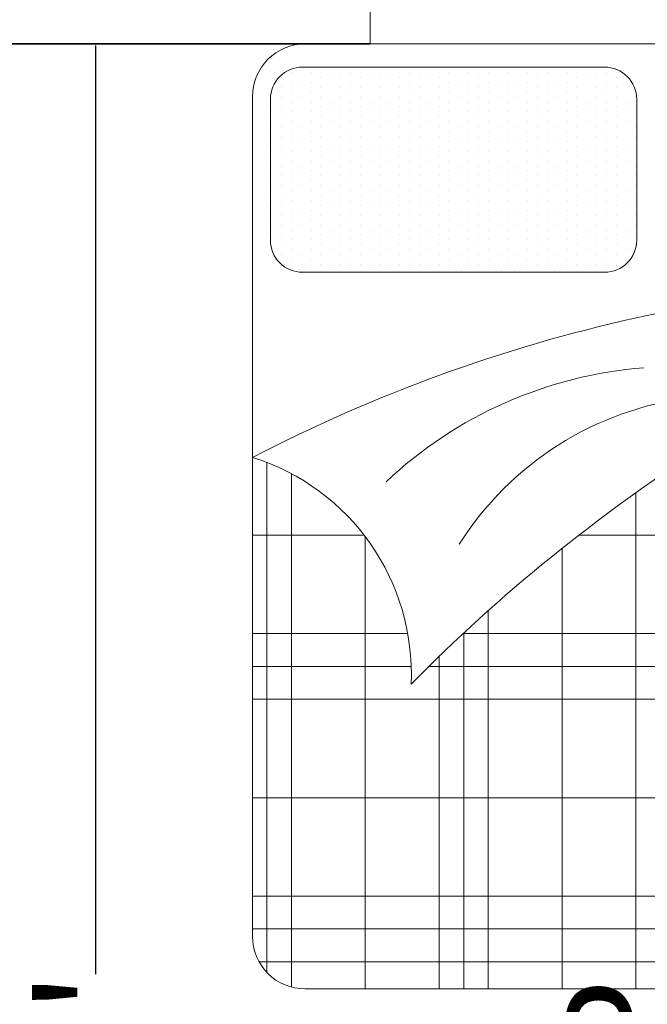
# Model space of a CAD drawing. Units: inches. Extents: x -269 to 4574, y -694 to 313.
# Tile 12 of 19: x 302 to 357, y -74 to 11. Entities that reach past the tile are written whole.
import ezdxf

# ---------------------------------------------------------------- set-up
doc = ezdxf.new("R2010")
doc.units = ezdxf.units.IN
doc.header["$MEASUREMENT"] = 0
for name, color, linetype, lineweight in [('A-FURN', 2, 'Continuous', 18), ('DIMENSION', 5, 'Continuous', 18), ('WALL', 1, 'Continuous', 35), ('WINDOWS', 2, 'Continuous', 18)]:
    doc.layers.add(name, color=color, linetype=linetype, lineweight=lineweight)
doc.dimstyles.get("Standard").update_dxf_attribs({"dimtxt": 10, "dimasz": 0.18, "dimexe": 0.18, "dimexo": 0.0625, "dimgap": 0.09, "dimtad": 0, "dimdec": 1, "dimzin": 0, "dimdsep": 46, "dimlunit": 3, "dimtxsty": 'Standard', "dimcen": 0.09, "dimclrt": 7, "dimadec": 0, "dimazin": 0, "dimtfac": 1, "dimtdec": 1, "dimtofl": 0, "dimtmove": 0, "dimatfit": 3, "dimfxl": 1, "dimtolj": 1, "dimtzin": 0, "dimarcsym": 0})

# ---------------------------------------------------------------- blocks, each defined once
blk = doc.blocks.new('*X12')
at = {"color": 0}
for p, q in [((266.25, 456.9375), (266.25, 456.9375)), ((266.4375, 457.03125), (266.4375, 457.03125)), ((266.625, 456.9375), (266.625, 456.9375)), ((266.8125, 457.03125), (266.8125, 457.03125)), ((267, 456.9375), (267, 456.9375)), ((267.1875, 457.03125), (267.1875, 457.03125)), ((267.375, 456.9375), (267.375, 456.9375)), ((267.5625, 457.03125), (267.5625, 457.03125)), ((267.75, 456.9375), (267.75, 456.9375)), ((267.9375, 457.03125), (267.9375, 457.03125)), ((268.125, 456.9375), (268.125, 456.9375)), ((268.3125, 457.03125), (268.3125, 457.03125)), ((268.5, 456.9375), (268.5, 456.9375)), ((268.6875, 457.03125), (268.6875, 457.03125)), ((268.875, 456.9375), (268.875, 456.9375)), ((269.0625, 457.03125), (269.0625, 457.03125)), ((269.25, 456.9375), (269.25, 456.9375)), ((269.4375, 457.03125), (269.4375, 457.03125)), ((269.625, 456.9375), (269.625, 456.9375)), ((269.8125, 457.03125), (269.8125, 457.03125)), ((270, 456.9375), (270, 456.9375)), ((270.1875, 457.03125), (270.1875, 457.03125)), ((270.375, 456.9375), (270.375, 456.9375)), ((270.5625, 457.03125), (270.5625, 457.03125)), ((270.75, 456.9375), (270.75, 456.9375)), ((270.9375, 457.03125), (270.9375, 457.03125)), ((271.125, 456.9375), (271.125, 456.9375)), ((271.3125, 457.03125), (271.3125, 457.03125)), ((271.5, 456.9375), (271.5, 456.9375)), ((271.6875, 457.03125), (271.6875, 457.03125)), ((271.875, 456.9375), (271.875, 456.9375)), ((272.0625, 457.03125), (272.0625, 457.03125)), ((272.25, 456.9375), (272.25, 456.9375)), ((266.0625, 456.84375), (266.0625, 456.84375)), ((266.25, 456.75), (266.25, 456.75)), ((266.4375, 456.84375), (266.4375, 456.84375)), ((266.625, 456.75), (266.625, 456.75)), ((266.8125, 456.84375), (266.8125, 456.84375)), ((267, 456.75), (267, 456.75)), ((267.1875, 456.84375), (267.1875, 456.84375)), ((267.375, 456.75), (267.375, 456.75)), ((267.5625, 456.84375), (267.5625, 456.84375)), ((267.75, 456.75), (267.75, 456.75)), ((267.9375, 456.84375), (267.9375, 456.84375)), ((268.125, 456.75), (268.125, 456.75)), ((268.3125, 456.84375), (268.3125, 456.84375)), ((268.5, 456.75), (268.5, 456.75)), ((268.6875, 456.84375), (268.6875, 456.84375)), ((268.875, 456.75), (268.875, 456.75)), ((269.0625, 456.84375), (269.0625, 456.84375)), ((269.25, 456.75), (269.25, 456.75)), ((269.4375, 456.84375), (269.4375, 456.84375)), ((269.625, 456.75), (269.625, 456.75)), ((269.8125, 456.84375), (269.8125, 456.84375)), ((270, 456.75), (270, 456.75)), ((270.1875, 456.84375), (270.1875, 456.84375)), ((270.375, 456.75), (270.375, 456.75)), ((270.5625, 456.84375), (270.5625, 456.84375)), ((270.75, 456.75), (270.75, 456.75)), ((270.9375, 456.84375), (270.9375, 456.84375)), ((271.125, 456.75), (271.125, 456.75)), ((271.3125, 456.84375), (271.3125, 456.84375)), ((271.5, 456.75), (271.5, 456.75)), ((271.6875, 456.84375), (271.6875, 456.84375)), ((271.875, 456.75), (271.875, 456.75)), ((272.0625, 456.84375), (272.0625, 456.84375)), ((272.25, 456.75), (272.25, 456.75)), ((272.4375, 456.84375), (272.4375, 456.84375)), ((272.625, 456.75), (272.625, 456.75)), ((265.875, 456.5625), (265.875, 456.5625)), ((266.0625, 456.65625), (266.0625, 456.65625)), ((266.25, 456.5625), (266.25, 456.5625)), ((266.4375, 456.65625), (266.4375, 456.65625)), ((266.625, 456.5625), (266.625, 456.5625)), ((266.8125, 456.65625), (266.8125, 456.65625)), ((267, 456.5625), (267, 456.5625)), ((267.1875, 456.65625), (267.1875, 456.65625)), ((267.375, 456.5625), (267.375, 456.5625)), ((267.5625, 456.65625), (267.5625, 456.65625)), ((267.75, 456.5625), (267.75, 456.5625)), ((267.9375, 456.65625), (267.9375, 456.65625)), ((268.125, 456.5625), (268.125, 456.5625)), ((268.3125, 456.65625), (268.3125, 456.65625)), ((268.5, 456.5625), (268.5, 456.5625)), ((268.6875, 456.65625), (268.6875, 456.65625)), ((268.875, 456.5625), (268.875, 456.5625)), ((269.0625, 456.65625), (269.0625, 456.65625)), ((269.25, 456.5625), (269.25, 456.5625)), ((269.4375, 456.65625), (269.4375, 456.65625)), ((269.625, 456.5625), (269.625, 456.5625)), ((269.8125, 456.65625), (269.8125, 456.65625)), ((270, 456.5625), (270, 456.5625)), ((270.1875, 456.65625), (270.1875, 456.65625)), ((270.375, 456.5625), (270.375, 456.5625)), ((270.5625, 456.65625), (270.5625, 456.65625)), ((270.75, 456.5625), (270.75, 456.5625)), ((270.9375, 456.65625), (270.9375, 456.65625)), ((271.125, 456.5625), (271.125, 456.5625)), ((271.3125, 456.65625), (271.3125, 456.65625)), ((271.5, 456.5625), (271.5, 456.5625)), ((271.6875, 456.65625), (271.6875, 456.65625)), ((271.875, 456.5625), (271.875, 456.5625)), ((272.0625, 456.65625), (272.0625, 456.65625)), ((272.25, 456.5625), (272.25, 456.5625)), ((272.4375, 456.65625), (272.4375, 456.65625)), ((272.625, 456.5625), (272.625, 456.5625)), ((265.875, 456.375), (265.875, 456.375)), ((266.0625, 456.46875), (266.0625, 456.46875)), ((266.25, 456.375), (266.25, 456.375)), ((266.4375, 456.46875), (266.4375, 456.46875)), ((266.625, 456.375), (266.625, 456.375)), ((266.8125, 456.46875), (266.8125, 456.46875)), ((267, 456.375), (267, 456.375)), ((267.1875, 456.46875), (267.1875, 456.46875)), ((267.375, 456.375), (267.375, 456.375)), ((267.5625, 456.46875), (267.5625, 456.46875)), ((267.75, 456.375), (267.75, 456.375)), ((267.9375, 456.46875), (267.9375, 456.46875)), ((268.125, 456.375), (268.125, 456.375)), ((268.3125, 456.46875), (268.3125, 456.46875)), ((268.5, 456.375), (268.5, 456.375)), ((268.6875, 456.46875), (268.6875, 456.46875)), ((268.875, 456.375), (268.875, 456.375)), ((269.0625, 456.46875), (269.0625, 456.46875)), ((269.25, 456.375), (269.25, 456.375)), ((269.4375, 456.46875), (269.4375, 456.46875)), ((269.625, 456.375), (269.625, 456.375)), ((269.8125, 456.46875), (269.8125, 456.46875)), ((270, 456.375), (270, 456.375)), ((270.1875, 456.46875), (270.1875, 456.46875)), ((270.375, 456.375), (270.375, 456.375)), ((270.5625, 456.46875), (270.5625, 456.46875)), ((270.75, 456.375), (270.75, 456.375)), ((270.9375, 456.46875), (270.9375, 456.46875)), ((271.125, 456.375), (271.125, 456.375)), ((271.3125, 456.46875), (271.3125, 456.46875)), ((271.5, 456.375), (271.5, 456.375)), ((271.6875, 456.46875), (271.6875, 456.46875)), ((271.875, 456.375), (271.875, 456.375)), ((272.0625, 456.46875), (272.0625, 456.46875)), ((272.25, 456.375), (272.25, 456.375)), ((272.4375, 456.46875), (272.4375, 456.46875)), ((272.625, 456.375), (272.625, 456.375)), ((272.8125, 456.46875), (272.8125, 456.46875)), ((265.875, 456.1875), (265.875, 456.1875)), ((266.0625, 456.28125), (266.0625, 456.28125)), ((266.25, 456.1875), (266.25, 456.1875)), ((266.4375, 456.28125), (266.4375, 456.28125)), ((266.625, 456.1875), (266.625, 456.1875)), ((266.8125, 456.28125), (266.8125, 456.28125)), ((267, 456.1875), (267, 456.1875)), ((267.1875, 456.28125), (267.1875, 456.28125)), ((267.375, 456.1875), (267.375, 456.1875)), ((267.5625, 456.28125), (267.5625, 456.28125)), ((267.75, 456.1875), (267.75, 456.1875)), ((267.9375, 456.28125), (267.9375, 456.28125)), ((268.125, 456.1875), (268.125, 456.1875)), ((268.3125, 456.28125), (268.3125, 456.28125)), ((268.5, 456.1875), (268.5, 456.1875)), ((268.6875, 456.28125), (268.6875, 456.28125)), ((268.875, 456.1875), (268.875, 456.1875)), ((269.0625, 456.28125), (269.0625, 456.28125)), ((269.25, 456.1875), (269.25, 456.1875)), ((269.4375, 456.28125), (269.4375, 456.28125)), ((269.625, 456.1875), (269.625, 456.1875)), ((269.8125, 456.28125), (269.8125, 456.28125)), ((270, 456.1875), (270, 456.1875)), ((270.1875, 456.28125), (270.1875, 456.28125)), ((270.375, 456.1875), (270.375, 456.1875)), ((270.5625, 456.28125), (270.5625, 456.28125)), ((270.75, 456.1875), (270.75, 456.1875)), ((270.9375, 456.28125), (270.9375, 456.28125)), ((271.125, 456.1875), (271.125, 456.1875)), ((271.3125, 456.28125), (271.3125, 456.28125)), ((271.5, 456.1875), (271.5, 456.1875)), ((271.6875, 456.28125), (271.6875, 456.28125)), ((271.875, 456.1875), (271.875, 456.1875)), ((272.0625, 456.28125), (272.0625, 456.28125)), ((272.25, 456.1875), (272.25, 456.1875)), ((272.4375, 456.28125), (272.4375, 456.28125)), ((272.625, 456.1875), (272.625, 456.1875)), ((272.8125, 456.28125), (272.8125, 456.28125)), ((265.875, 456), (265.875, 456)), ((266.0625, 456.09375), (266.0625, 456.09375)), ((266.25, 456), (266.25, 456)), ((266.4375, 456.09375), (266.4375, 456.09375)), ((266.625, 456), (266.625, 456)), ((266.8125, 456.09375), (266.8125, 456.09375)), ((267, 456), (267, 456)), ((267.1875, 456.09375), (267.1875, 456.09375)), ((267.375, 456), (267.375, 456)), ((267.5625, 456.09375), (267.5625, 456.09375)), ((267.75, 456), (267.75, 456)), ((267.9375, 456.09375), (267.9375, 456.09375)), ((268.125, 456), (268.125, 456)), ((268.3125, 456.09375), (268.3125, 456.09375)), ((268.5, 456), (268.5, 456)), ((268.6875, 456.09375), (268.6875, 456.09375)), ((268.875, 456), (268.875, 456)), ((269.0625, 456.09375), (269.0625, 456.09375)), ((269.25, 456), (269.25, 456)), ((269.4375, 456.09375), (269.4375, 456.09375)), ((269.625, 456), (269.625, 456)), ((269.8125, 456.09375), (269.8125, 456.09375)), ((270, 456), (270, 456)), ((270.1875, 456.09375), (270.1875, 456.09375)), ((270.375, 456), (270.375, 456)), ((270.5625, 456.09375), (270.5625, 456.09375)), ((270.75, 456), (270.75, 456)), ((270.9375, 456.09375), (270.9375, 456.09375)), ((271.125, 456), (271.125, 456)), ((271.3125, 456.09375), (271.3125, 456.09375)), ((271.5, 456), (271.5, 456)), ((271.6875, 456.09375), (271.6875, 456.09375)), ((271.875, 456), (271.875, 456)), ((272.0625, 456.09375), (272.0625, 456.09375)), ((272.25, 456), (272.25, 456)), ((272.4375, 456.09375), (272.4375, 456.09375)), ((272.625, 456), (272.625, 456)), ((272.8125, 456.09375), (272.8125, 456.09375)), ((265.875, 455.8125), (265.875, 455.8125)), ((266.0625, 455.90625), (266.0625, 455.90625)), ((266.25, 455.8125), (266.25, 455.8125)), ((266.4375, 455.90625), (266.4375, 455.90625)), ((266.625, 455.8125), (266.625, 455.8125)), ((266.8125, 455.90625), (266.8125, 455.90625)), ((267, 455.8125), (267, 455.8125)), ((267.1875, 455.90625), (267.1875, 455.90625)), ((267.375, 455.8125), (267.375, 455.8125)), ((267.5625, 455.90625), (267.5625, 455.90625)), ((267.75, 455.8125), (267.75, 455.8125)), ((267.9375, 455.90625), (267.9375, 455.90625)), ((268.125, 455.8125), (268.125, 455.8125)), ((268.3125, 455.90625), (268.3125, 455.90625)), ((268.5, 455.8125), (268.5, 455.8125)), ((268.6875, 455.90625), (268.6875, 455.90625)), ((268.875, 455.8125), (268.875, 455.8125)), ((269.0625, 455.90625), (269.0625, 455.90625)), ((269.25, 455.8125), (269.25, 455.8125)), ((269.4375, 455.90625), (269.4375, 455.90625)), ((269.625, 455.8125), (269.625, 455.8125)), ((269.8125, 455.90625), (269.8125, 455.90625)), ((270, 455.8125), (270, 455.8125)), ((270.1875, 455.90625), (270.1875, 455.90625)), ((270.375, 455.8125), (270.375, 455.8125)), ((270.5625, 455.90625), (270.5625, 455.90625)), ((270.75, 455.8125), (270.75, 455.8125)), ((270.9375, 455.90625), (270.9375, 455.90625)), ((271.125, 455.8125), (271.125, 455.8125)), ((271.3125, 455.90625), (271.3125, 455.90625)), ((271.5, 455.8125), (271.5, 455.8125)), ((271.6875, 455.90625), (271.6875, 455.90625)), ((271.875, 455.8125), (271.875, 455.8125)), ((272.0625, 455.90625), (272.0625, 455.90625)), ((272.25, 455.8125), (272.25, 455.8125)), ((272.4375, 455.90625), (272.4375, 455.90625)), ((272.625, 455.8125), (272.625, 455.8125)), ((272.8125, 455.90625), (272.8125, 455.90625)), ((265.875, 455.625), (265.875, 455.625)), ((266.0625, 455.71875), (266.0625, 455.71875)), ((266.25, 455.625), (266.25, 455.625)), ((266.4375, 455.71875), (266.4375, 455.71875)), ((266.625, 455.625), (266.625, 455.625)), ((266.8125, 455.71875), (266.8125, 455.71875)), ((267, 455.625), (267, 455.625)), ((267.1875, 455.71875), (267.1875, 455.71875)), ((267.375, 455.625), (267.375, 455.625)), ((267.5625, 455.71875), (267.5625, 455.71875)), ((267.75, 455.625), (267.75, 455.625)), ((267.9375, 455.71875), (267.9375, 455.71875)), ((268.125, 455.625), (268.125, 455.625)), ((268.3125, 455.71875), (268.3125, 455.71875)), ((268.5, 455.625), (268.5, 455.625)), ((268.6875, 455.71875), (268.6875, 455.71875)), ((268.875, 455.625), (268.875, 455.625)), ((269.0625, 455.71875), (269.0625, 455.71875)), ((269.25, 455.625), (269.25, 455.625)), ((269.4375, 455.71875), (269.4375, 455.71875)), ((269.625, 455.625), (269.625, 455.625)), ((269.8125, 455.71875), (269.8125, 455.71875)), ((270, 455.625), (270, 455.625)), ((270.1875, 455.71875), (270.1875, 455.71875)), ((270.375, 455.625), (270.375, 455.625)), ((270.5625, 455.71875), (270.5625, 455.71875)), ((270.75, 455.625), (270.75, 455.625)), ((270.9375, 455.71875), (270.9375, 455.71875)), ((271.125, 455.625), (271.125, 455.625)), ((271.3125, 455.71875), (271.3125, 455.71875)), ((271.5, 455.625), (271.5, 455.625)), ((271.6875, 455.71875), (271.6875, 455.71875)), ((271.875, 455.625), (271.875, 455.625)), ((272.0625, 455.71875), (272.0625, 455.71875)), ((272.25, 455.625), (272.25, 455.625)), ((272.4375, 455.71875), (272.4375, 455.71875)), ((272.625, 455.625), (272.625, 455.625)), ((272.8125, 455.71875), (272.8125, 455.71875)), ((265.875, 455.4375), (265.875, 455.4375)), ((266.0625, 455.53125), (266.0625, 455.53125)), ((266.25, 455.4375), (266.25, 455.4375)), ((266.4375, 455.53125), (266.4375, 455.53125)), ((266.625, 455.4375), (266.625, 455.4375)), ((266.8125, 455.53125), (266.8125, 455.53125)), ((267, 455.4375), (267, 455.4375)), ((267.1875, 455.53125), (267.1875, 455.53125)), ((267.375, 455.4375), (267.375, 455.4375)), ((267.5625, 455.53125), (267.5625, 455.53125)), ((267.75, 455.4375), (267.75, 455.4375)), ((267.9375, 455.53125), (267.9375, 455.53125)), ((268.125, 455.4375), (268.125, 455.4375)), ((268.3125, 455.53125), (268.3125, 455.53125)), ((268.5, 455.4375), (268.5, 455.4375)), ((268.6875, 455.53125), (268.6875, 455.53125)), ((268.875, 455.4375), (268.875, 455.4375)), ((269.0625, 455.53125), (269.0625, 455.53125)), ((269.25, 455.4375), (269.25, 455.4375)), ((269.4375, 455.53125), (269.4375, 455.53125)), ((269.625, 455.4375), (269.625, 455.4375)), ((269.8125, 455.53125), (269.8125, 455.53125)), ((270, 455.4375), (270, 455.4375)), ((270.1875, 455.53125), (270.1875, 455.53125)), ((270.375, 455.4375), (270.375, 455.4375)), ((270.5625, 455.53125), (270.5625, 455.53125)), ((270.75, 455.4375), (270.75, 455.4375)), ((270.9375, 455.53125), (270.9375, 455.53125)), ((271.125, 455.4375), (271.125, 455.4375)), ((271.3125, 455.53125), (271.3125, 455.53125)), ((271.5, 455.4375), (271.5, 455.4375)), ((271.6875, 455.53125), (271.6875, 455.53125)), ((271.875, 455.4375), (271.875, 455.4375)), ((272.0625, 455.53125), (272.0625, 455.53125)), ((272.25, 455.4375), (272.25, 455.4375)), ((272.4375, 455.53125), (272.4375, 455.53125)), ((272.625, 455.4375), (272.625, 455.4375)), ((272.8125, 455.53125), (272.8125, 455.53125)), ((265.875, 455.25), (265.875, 455.25)), ((266.0625, 455.34375), (266.0625, 455.34375)), ((266.25, 455.25), (266.25, 455.25)), ((266.4375, 455.34375), (266.4375, 455.34375)), ((266.625, 455.25), (266.625, 455.25)), ((266.8125, 455.34375), (266.8125, 455.34375)), ((267, 455.25), (267, 455.25)), ((267.1875, 455.34375), (267.1875, 455.34375)), ((267.375, 455.25), (267.375, 455.25)), ((267.5625, 455.34375), (267.5625, 455.34375)), ((267.75, 455.25), (267.75, 455.25)), ((267.9375, 455.34375), (267.9375, 455.34375)), ((268.125, 455.25), (268.125, 455.25)), ((268.3125, 455.34375), (268.3125, 455.34375)), ((268.5, 455.25), (268.5, 455.25)), ((268.6875, 455.34375), (268.6875, 455.34375)), ((268.875, 455.25), (268.875, 455.25)), ((269.0625, 455.34375), (269.0625, 455.34375)), ((269.25, 455.25), (269.25, 455.25)), ((269.4375, 455.34375), (269.4375, 455.34375)), ((269.625, 455.25), (269.625, 455.25)), ((269.8125, 455.34375), (269.8125, 455.34375)), ((270, 455.25), (270, 455.25)), ((270.1875, 455.34375), (270.1875, 455.34375)), ((270.375, 455.25), (270.375, 455.25)), ((270.5625, 455.34375), (270.5625, 455.34375)), ((270.75, 455.25), (270.75, 455.25)), ((270.9375, 455.34375), (270.9375, 455.34375)), ((271.125, 455.25), (271.125, 455.25)), ((271.3125, 455.34375), (271.3125, 455.34375)), ((271.5, 455.25), (271.5, 455.25)), ((271.6875, 455.34375), (271.6875, 455.34375)), ((271.875, 455.25), (271.875, 455.25)), ((272.0625, 455.34375), (272.0625, 455.34375)), ((272.25, 455.25), (272.25, 455.25)), ((272.4375, 455.34375), (272.4375, 455.34375)), ((272.625, 455.25), (272.625, 455.25)), ((272.8125, 455.34375), (272.8125, 455.34375)), ((265.875, 455.0625), (265.875, 455.0625)), ((266.0625, 455.15625), (266.0625, 455.15625)), ((266.25, 455.0625), (266.25, 455.0625)), ((266.4375, 455.15625), (266.4375, 455.15625)), ((266.625, 455.0625), (266.625, 455.0625)), ((266.8125, 455.15625), (266.8125, 455.15625)), ((267, 455.0625), (267, 455.0625)), ((267.1875, 455.15625), (267.1875, 455.15625)), ((267.375, 455.0625), (267.375, 455.0625)), ((267.5625, 455.15625), (267.5625, 455.15625)), ((267.75, 455.0625), (267.75, 455.0625)), ((267.9375, 455.15625), (267.9375, 455.15625)), ((268.125, 455.0625), (268.125, 455.0625)), ((268.3125, 455.15625), (268.3125, 455.15625)), ((268.5, 455.0625), (268.5, 455.0625)), ((268.6875, 455.15625), (268.6875, 455.15625)), ((268.875, 455.0625), (268.875, 455.0625)), ((269.0625, 455.15625), (269.0625, 455.15625)), ((269.25, 455.0625), (269.25, 455.0625)), ((269.4375, 455.15625), (269.4375, 455.15625)), ((269.625, 455.0625), (269.625, 455.0625)), ((269.8125, 455.15625), (269.8125, 455.15625)), ((270, 455.0625), (270, 455.0625)), ((270.1875, 455.15625), (270.1875, 455.15625)), ((270.375, 455.0625), (270.375, 455.0625)), ((270.5625, 455.15625), (270.5625, 455.15625)), ((270.75, 455.0625), (270.75, 455.0625)), ((270.9375, 455.15625), (270.9375, 455.15625)), ((271.125, 455.0625), (271.125, 455.0625)), ((271.3125, 455.15625), (271.3125, 455.15625)), ((271.5, 455.0625), (271.5, 455.0625)), ((271.6875, 455.15625), (271.6875, 455.15625)), ((271.875, 455.0625), (271.875, 455.0625)), ((272.0625, 455.15625), (272.0625, 455.15625)), ((272.25, 455.0625), (272.25, 455.0625)), ((272.4375, 455.15625), (272.4375, 455.15625)), ((272.625, 455.0625), (272.625, 455.0625)), ((272.8125, 455.15625), (272.8125, 455.15625)), ((265.875, 454.875), (265.875, 454.875)), ((266.0625, 454.96875), (266.0625, 454.96875)), ((266.25, 454.875), (266.25, 454.875)), ((266.4375, 454.96875), (266.4375, 454.96875)), ((266.625, 454.875), (266.625, 454.875)), ((266.8125, 454.96875), (266.8125, 454.96875)), ((267, 454.875), (267, 454.875)), ((267.1875, 454.96875), (267.1875, 454.96875)), ((267.375, 454.875), (267.375, 454.875)), ((267.5625, 454.96875), (267.5625, 454.96875)), ((267.75, 454.875), (267.75, 454.875)), ((267.9375, 454.96875), (267.9375, 454.96875)), ((268.125, 454.875), (268.125, 454.875)), ((268.3125, 454.96875), (268.3125, 454.96875)), ((268.5, 454.875), (268.5, 454.875)), ((268.6875, 454.96875), (268.6875, 454.96875)), ((268.875, 454.875), (268.875, 454.875)), ((269.0625, 454.96875), (269.0625, 454.96875)), ((269.25, 454.875), (269.25, 454.875)), ((269.4375, 454.96875), (269.4375, 454.96875)), ((269.625, 454.875), (269.625, 454.875)), ((269.8125, 454.96875), (269.8125, 454.96875)), ((270, 454.875), (270, 454.875)), ((270.1875, 454.96875), (270.1875, 454.96875)), ((270.375, 454.875), (270.375, 454.875)), ((270.5625, 454.96875), (270.5625, 454.96875)), ((270.75, 454.875), (270.75, 454.875)), ((270.9375, 454.96875), (270.9375, 454.96875)), ((271.125, 454.875), (271.125, 454.875)), ((271.3125, 454.96875), (271.3125, 454.96875)), ((271.5, 454.875), (271.5, 454.875)), ((271.6875, 454.96875), (271.6875, 454.96875)), ((271.875, 454.875), (271.875, 454.875)), ((272.0625, 454.96875), (272.0625, 454.96875)), ((272.25, 454.875), (272.25, 454.875)), ((272.4375, 454.96875), (272.4375, 454.96875)), ((272.625, 454.875), (272.625, 454.875)), ((272.8125, 454.96875), (272.8125, 454.96875)), ((265.875, 454.6875), (265.875, 454.6875)), ((266.0625, 454.78125), (266.0625, 454.78125)), ((266.25, 454.6875), (266.25, 454.6875)), ((266.4375, 454.78125), (266.4375, 454.78125)), ((266.625, 454.6875), (266.625, 454.6875)), ((266.8125, 454.78125), (266.8125, 454.78125)), ((267, 454.6875), (267, 454.6875)), ((267.1875, 454.78125), (267.1875, 454.78125)), ((267.375, 454.6875), (267.375, 454.6875)), ((267.5625, 454.78125), (267.5625, 454.78125)), ((267.75, 454.6875), (267.75, 454.6875)), ((267.9375, 454.78125), (267.9375, 454.78125)), ((268.125, 454.6875), (268.125, 454.6875)), ((268.3125, 454.78125), (268.3125, 454.78125)), ((268.5, 454.6875), (268.5, 454.6875)), ((268.6875, 454.78125), (268.6875, 454.78125)), ((268.875, 454.6875), (268.875, 454.6875)), ((269.0625, 454.78125), (269.0625, 454.78125)), ((269.25, 454.6875), (269.25, 454.6875)), ((269.4375, 454.78125), (269.4375, 454.78125)), ((269.625, 454.6875), (269.625, 454.6875)), ((269.8125, 454.78125), (269.8125, 454.78125)), ((270, 454.6875), (270, 454.6875)), ((270.1875, 454.78125), (270.1875, 454.78125)), ((270.375, 454.6875), (270.375, 454.6875)), ((270.5625, 454.78125), (270.5625, 454.78125)), ((270.75, 454.6875), (270.75, 454.6875)), ((270.9375, 454.78125), (270.9375, 454.78125)), ((271.125, 454.6875), (271.125, 454.6875)), ((271.3125, 454.78125), (271.3125, 454.78125)), ((271.5, 454.6875), (271.5, 454.6875)), ((271.6875, 454.78125), (271.6875, 454.78125)), ((271.875, 454.6875), (271.875, 454.6875)), ((272.0625, 454.78125), (272.0625, 454.78125)), ((272.25, 454.6875), (272.25, 454.6875)), ((272.4375, 454.78125), (272.4375, 454.78125)), ((272.625, 454.6875), (272.625, 454.6875)), ((272.8125, 454.78125), (272.8125, 454.78125)), ((265.875, 454.5), (265.875, 454.5)), ((266.0625, 454.59375), (266.0625, 454.59375)), ((266.25, 454.5), (266.25, 454.5)), ((266.4375, 454.59375), (266.4375, 454.59375)), ((266.625, 454.5), (266.625, 454.5)), ((266.8125, 454.59375), (266.8125, 454.59375)), ((267, 454.5), (267, 454.5)), ((267.1875, 454.59375), (267.1875, 454.59375)), ((267.375, 454.5), (267.375, 454.5)), ((267.5625, 454.59375), (267.5625, 454.59375)), ((267.75, 454.5), (267.75, 454.5)), ((267.9375, 454.59375), (267.9375, 454.59375)), ((268.125, 454.5), (268.125, 454.5)), ((268.3125, 454.59375), (268.3125, 454.59375)), ((268.5, 454.5), (268.5, 454.5)), ((268.6875, 454.59375), (268.6875, 454.59375)), ((268.875, 454.5), (268.875, 454.5)), ((269.0625, 454.59375), (269.0625, 454.59375)), ((269.25, 454.5), (269.25, 454.5)), ((269.4375, 454.59375), (269.4375, 454.59375)), ((269.625, 454.5), (269.625, 454.5)), ((269.8125, 454.59375), (269.8125, 454.59375)), ((270, 454.5), (270, 454.5)), ((270.1875, 454.59375), (270.1875, 454.59375)), ((270.375, 454.5), (270.375, 454.5)), ((270.5625, 454.59375), (270.5625, 454.59375)), ((270.75, 454.5), (270.75, 454.5)), ((270.9375, 454.59375), (270.9375, 454.59375)), ((271.125, 454.5), (271.125, 454.5)), ((271.3125, 454.59375), (271.3125, 454.59375)), ((271.5, 454.5), (271.5, 454.5)), ((271.6875, 454.59375), (271.6875, 454.59375)), ((271.875, 454.5), (271.875, 454.5)), ((272.0625, 454.59375), (272.0625, 454.59375)), ((272.25, 454.5), (272.25, 454.5)), ((272.4375, 454.59375), (272.4375, 454.59375)), ((272.625, 454.5), (272.625, 454.5)), ((272.8125, 454.59375), (272.8125, 454.59375)), ((265.875, 454.3125), (265.875, 454.3125)), ((266.0625, 454.40625), (266.0625, 454.40625)), ((266.25, 454.3125), (266.25, 454.3125)), ((266.4375, 454.40625), (266.4375, 454.40625)), ((266.625, 454.3125), (266.625, 454.3125)), ((266.8125, 454.40625), (266.8125, 454.40625)), ((267, 454.3125), (267, 454.3125)), ((267.1875, 454.40625), (267.1875, 454.40625)), ((267.375, 454.3125), (267.375, 454.3125)), ((267.5625, 454.40625), (267.5625, 454.40625)), ((267.75, 454.3125), (267.75, 454.3125)), ((267.9375, 454.40625), (267.9375, 454.40625)), ((268.125, 454.3125), (268.125, 454.3125)), ((268.3125, 454.40625), (268.3125, 454.40625)), ((268.5, 454.3125), (268.5, 454.3125)), ((268.6875, 454.40625), (268.6875, 454.40625)), ((268.875, 454.3125), (268.875, 454.3125)), ((269.0625, 454.40625), (269.0625, 454.40625)), ((269.25, 454.3125), (269.25, 454.3125)), ((269.4375, 454.40625), (269.4375, 454.40625)), ((269.625, 454.3125), (269.625, 454.3125)), ((269.8125, 454.40625), (269.8125, 454.40625)), ((270, 454.3125), (270, 454.3125)), ((270.1875, 454.40625), (270.1875, 454.40625)), ((270.375, 454.3125), (270.375, 454.3125)), ((270.5625, 454.40625), (270.5625, 454.40625)), ((270.75, 454.3125), (270.75, 454.3125)), ((270.9375, 454.40625), (270.9375, 454.40625)), ((271.125, 454.3125), (271.125, 454.3125)), ((271.3125, 454.40625), (271.3125, 454.40625)), ((271.5, 454.3125), (271.5, 454.3125)), ((271.6875, 454.40625), (271.6875, 454.40625)), ((271.875, 454.3125), (271.875, 454.3125)), ((272.0625, 454.40625), (272.0625, 454.40625)), ((272.25, 454.3125), (272.25, 454.3125)), ((272.4375, 454.40625), (272.4375, 454.40625)), ((272.625, 454.3125), (272.625, 454.3125)), ((272.8125, 454.40625), (272.8125, 454.40625)), ((265.875, 454.125), (265.875, 454.125)), ((266.0625, 454.21875), (266.0625, 454.21875)), ((266.25, 454.125), (266.25, 454.125)), ((266.4375, 454.21875), (266.4375, 454.21875)), ((266.625, 454.125), (266.625, 454.125)), ((266.8125, 454.21875), (266.8125, 454.21875)), ((267, 454.125), (267, 454.125)), ((267.1875, 454.21875), (267.1875, 454.21875)), ((267.375, 454.125), (267.375, 454.125)), ((267.5625, 454.21875), (267.5625, 454.21875)), ((267.75, 454.125), (267.75, 454.125)), ((267.9375, 454.21875), (267.9375, 454.21875)), ((268.125, 454.125), (268.125, 454.125)), ((268.3125, 454.21875), (268.3125, 454.21875)), ((268.5, 454.125), (268.5, 454.125)), ((268.6875, 454.21875), (268.6875, 454.21875)), ((268.875, 454.125), (268.875, 454.125)), ((269.0625, 454.21875), (269.0625, 454.21875)), ((269.25, 454.125), (269.25, 454.125)), ((269.4375, 454.21875), (269.4375, 454.21875)), ((269.625, 454.125), (269.625, 454.125)), ((269.8125, 454.21875), (269.8125, 454.21875)), ((270, 454.125), (270, 454.125)), ((270.1875, 454.21875), (270.1875, 454.21875)), ((270.375, 454.125), (270.375, 454.125)), ((270.5625, 454.21875), (270.5625, 454.21875)), ((270.75, 454.125), (270.75, 454.125)), ((270.9375, 454.21875), (270.9375, 454.21875)), ((271.125, 454.125), (271.125, 454.125)), ((271.3125, 454.21875), (271.3125, 454.21875)), ((271.5, 454.125), (271.5, 454.125)), ((271.6875, 454.21875), (271.6875, 454.21875)), ((271.875, 454.125), (271.875, 454.125)), ((272.0625, 454.21875), (272.0625, 454.21875)), ((272.25, 454.125), (272.25, 454.125)), ((272.4375, 454.21875), (272.4375, 454.21875)), ((272.625, 454.125), (272.625, 454.125)), ((272.8125, 454.21875), (272.8125, 454.21875)), ((265.875, 453.9375), (265.875, 453.9375)), ((266.0625, 454.03125), (266.0625, 454.03125)), ((266.25, 453.9375), (266.25, 453.9375)), ((266.4375, 454.03125), (266.4375, 454.03125)), ((266.625, 453.9375), (266.625, 453.9375)), ((266.8125, 454.03125), (266.8125, 454.03125)), ((267, 453.9375), (267, 453.9375)), ((267.1875, 454.03125), (267.1875, 454.03125)), ((267.375, 453.9375), (267.375, 453.9375)), ((267.5625, 454.03125), (267.5625, 454.03125)), ((267.75, 453.9375), (267.75, 453.9375)), ((267.9375, 454.03125), (267.9375, 454.03125)), ((268.125, 453.9375), (268.125, 453.9375)), ((268.3125, 454.03125), (268.3125, 454.03125)), ((268.5, 453.9375), (268.5, 453.9375)), ((268.6875, 454.03125), (268.6875, 454.03125)), ((268.875, 453.9375), (268.875, 453.9375)), ((269.0625, 454.03125), (269.0625, 454.03125)), ((269.25, 453.9375), (269.25, 453.9375)), ((269.4375, 454.03125), (269.4375, 454.03125)), ((269.625, 453.9375), (269.625, 453.9375)), ((269.8125, 454.03125), (269.8125, 454.03125)), ((270, 453.9375), (270, 453.9375)), ((270.1875, 454.03125), (270.1875, 454.03125)), ((270.375, 453.9375), (270.375, 453.9375)), ((270.5625, 454.03125), (270.5625, 454.03125)), ((270.75, 453.9375), (270.75, 453.9375)), ((270.9375, 454.03125), (270.9375, 454.03125)), ((271.125, 453.9375), (271.125, 453.9375)), ((271.3125, 454.03125), (271.3125, 454.03125)), ((271.5, 453.9375), (271.5, 453.9375)), ((271.6875, 454.03125), (271.6875, 454.03125)), ((271.875, 453.9375), (271.875, 453.9375)), ((272.0625, 454.03125), (272.0625, 454.03125)), ((272.25, 453.9375), (272.25, 453.9375)), ((272.4375, 454.03125), (272.4375, 454.03125)), ((272.625, 453.9375), (272.625, 453.9375)), ((272.8125, 454.03125), (272.8125, 454.03125)), ((265.875, 453.75), (265.875, 453.75)), ((266.0625, 453.84375), (266.0625, 453.84375)), ((266.25, 453.75), (266.25, 453.75)), ((266.4375, 453.84375), (266.4375, 453.84375)), ((266.625, 453.75), (266.625, 453.75)), ((266.8125, 453.84375), (266.8125, 453.84375)), ((267, 453.75), (267, 453.75)), ((267.1875, 453.84375), (267.1875, 453.84375)), ((267.375, 453.75), (267.375, 453.75)), ((267.5625, 453.84375), (267.5625, 453.84375)), ((267.75, 453.75), (267.75, 453.75)), ((267.9375, 453.84375), (267.9375, 453.84375)), ((268.125, 453.75), (268.125, 453.75)), ((268.3125, 453.84375), (268.3125, 453.84375)), ((268.5, 453.75), (268.5, 453.75)), ((268.6875, 453.84375), (268.6875, 453.84375)), ((268.875, 453.75), (268.875, 453.75)), ((269.0625, 453.84375), (269.0625, 453.84375)), ((269.25, 453.75), (269.25, 453.75)), ((269.4375, 453.84375), (269.4375, 453.84375)), ((269.625, 453.75), (269.625, 453.75)), ((269.8125, 453.84375), (269.8125, 453.84375)), ((270, 453.75), (270, 453.75)), ((270.1875, 453.84375), (270.1875, 453.84375)), ((270.375, 453.75), (270.375, 453.75)), ((270.5625, 453.84375), (270.5625, 453.84375)), ((270.75, 453.75), (270.75, 453.75)), ((270.9375, 453.84375), (270.9375, 453.84375)), ((271.125, 453.75), (271.125, 453.75)), ((271.3125, 453.84375), (271.3125, 453.84375)), ((271.5, 453.75), (271.5, 453.75)), ((271.6875, 453.84375), (271.6875, 453.84375)), ((271.875, 453.75), (271.875, 453.75)), ((272.0625, 453.84375), (272.0625, 453.84375)), ((272.25, 453.75), (272.25, 453.75)), ((272.4375, 453.84375), (272.4375, 453.84375)), ((272.625, 453.75), (272.625, 453.75)), ((272.8125, 453.84375), (272.8125, 453.84375)), ((266.0625, 453.65625), (266.0625, 453.65625)), ((266.25, 453.5625), (266.25, 453.5625)), ((266.4375, 453.65625), (266.4375, 453.65625)), ((266.625, 453.5625), (266.625, 453.5625)), ((266.8125, 453.65625), (266.8125, 453.65625)), ((267, 453.5625), (267, 453.5625)), ((267.1875, 453.65625), (267.1875, 453.65625)), ((267.375, 453.5625), (267.375, 453.5625)), ((267.5625, 453.65625), (267.5625, 453.65625)), ((267.75, 453.5625), (267.75, 453.5625)), ((267.9375, 453.65625), (267.9375, 453.65625)), ((268.125, 453.5625), (268.125, 453.5625)), ((268.3125, 453.65625), (268.3125, 453.65625)), ((268.5, 453.5625), (268.5, 453.5625)), ((268.6875, 453.65625), (268.6875, 453.65625)), ((268.875, 453.5625), (268.875, 453.5625)), ((269.0625, 453.65625), (269.0625, 453.65625)), ((269.25, 453.5625), (269.25, 453.5625)), ((269.4375, 453.65625), (269.4375, 453.65625)), ((269.625, 453.5625), (269.625, 453.5625)), ((269.8125, 453.65625), (269.8125, 453.65625)), ((270, 453.5625), (270, 453.5625)), ((270.1875, 453.65625), (270.1875, 453.65625)), ((270.375, 453.5625), (270.375, 453.5625)), ((270.5625, 453.65625), (270.5625, 453.65625)), ((270.75, 453.5625), (270.75, 453.5625)), ((270.9375, 453.65625), (270.9375, 453.65625)), ((271.125, 453.5625), (271.125, 453.5625)), ((271.3125, 453.65625), (271.3125, 453.65625)), ((271.5, 453.5625), (271.5, 453.5625)), ((271.6875, 453.65625), (271.6875, 453.65625)), ((271.875, 453.5625), (271.875, 453.5625)), ((272.0625, 453.65625), (272.0625, 453.65625)), ((272.25, 453.5625), (272.25, 453.5625)), ((272.4375, 453.65625), (272.4375, 453.65625)), ((272.625, 453.5625), (272.625, 453.5625)), ((272.8125, 453.65625), (272.8125, 453.65625)), ((266.0625, 453.46875), (266.0625, 453.46875)), ((266.25, 453.375), (266.25, 453.375)), ((266.4375, 453.46875), (266.4375, 453.46875)), ((266.625, 453.375), (266.625, 453.375)), ((266.8125, 453.46875), (266.8125, 453.46875)), ((267, 453.375), (267, 453.375)), ((267.1875, 453.46875), (267.1875, 453.46875)), ((267.375, 453.375), (267.375, 453.375)), ((267.5625, 453.46875), (267.5625, 453.46875)), ((267.75, 453.375), (267.75, 453.375)), ((267.9375, 453.46875), (267.9375, 453.46875)), ((268.125, 453.375), (268.125, 453.375)), ((268.3125, 453.46875), (268.3125, 453.46875)), ((268.5, 453.375), (268.5, 453.375)), ((268.6875, 453.46875), (268.6875, 453.46875)), ((268.875, 453.375), (268.875, 453.375)), ((269.0625, 453.46875), (269.0625, 453.46875)), ((269.25, 453.375), (269.25, 453.375)), ((269.4375, 453.46875), (269.4375, 453.46875)), ((269.625, 453.375), (269.625, 453.375)), ((269.8125, 453.46875), (269.8125, 453.46875)), ((270, 453.375), (270, 453.375)), ((270.1875, 453.46875), (270.1875, 453.46875)), ((270.375, 453.375), (270.375, 453.375)), ((270.5625, 453.46875), (270.5625, 453.46875)), ((270.75, 453.375), (270.75, 453.375)), ((270.9375, 453.46875), (270.9375, 453.46875)), ((271.125, 453.375), (271.125, 453.375)), ((271.3125, 453.46875), (271.3125, 453.46875)), ((271.5, 453.375), (271.5, 453.375)), ((271.6875, 453.46875), (271.6875, 453.46875)), ((271.875, 453.375), (271.875, 453.375)), ((272.0625, 453.46875), (272.0625, 453.46875)), ((272.25, 453.375), (272.25, 453.375)), ((272.4375, 453.46875), (272.4375, 453.46875)), ((272.625, 453.375), (272.625, 453.375)), ((266.0625, 453.28125), (266.0625, 453.28125)), ((266.25, 453.1875), (266.25, 453.1875)), ((266.4375, 453.28125), (266.4375, 453.28125)), ((266.625, 453.1875), (266.625, 453.1875)), ((266.8125, 453.28125), (266.8125, 453.28125)), ((267, 453.1875), (267, 453.1875)), ((267.1875, 453.28125), (267.1875, 453.28125)), ((267.375, 453.1875), (267.375, 453.1875)), ((267.5625, 453.28125), (267.5625, 453.28125)), ((267.75, 453.1875), (267.75, 453.1875)), ((267.9375, 453.28125), (267.9375, 453.28125)), ((268.125, 453.1875), (268.125, 453.1875)), ((268.3125, 453.28125), (268.3125, 453.28125)), ((268.5, 453.1875), (268.5, 453.1875)), ((268.6875, 453.28125), (268.6875, 453.28125)), ((268.875, 453.1875), (268.875, 453.1875)), ((269.0625, 453.28125), (269.0625, 453.28125)), ((269.25, 453.1875), (269.25, 453.1875)), ((269.4375, 453.28125), (269.4375, 453.28125)), ((269.625, 453.1875), (269.625, 453.1875)), ((269.8125, 453.28125), (269.8125, 453.28125)), ((270, 453.1875), (270, 453.1875)), ((270.1875, 453.28125), (270.1875, 453.28125)), ((270.375, 453.1875), (270.375, 453.1875)), ((270.5625, 453.28125), (270.5625, 453.28125)), ((270.75, 453.1875), (270.75, 453.1875)), ((270.9375, 453.28125), (270.9375, 453.28125)), ((271.125, 453.1875), (271.125, 453.1875)), ((271.3125, 453.28125), (271.3125, 453.28125)), ((271.5, 453.1875), (271.5, 453.1875)), ((271.6875, 453.28125), (271.6875, 453.28125)), ((271.875, 453.1875), (271.875, 453.1875)), ((272.0625, 453.28125), (272.0625, 453.28125)), ((272.25, 453.1875), (272.25, 453.1875)), ((272.4375, 453.28125), (272.4375, 453.28125))]:
    blk.add_line(p, q, dxfattribs=at)
blk = doc.blocks.new('*D19')
at = {"layer": 'Defpoints', "color": 0, "lineweight": 0, "transparency": 16777216}
for p in [(308.758, 9.268), (313.445, 9.268), (313.445, -170.732)]:
    blk.add_point(p, dxfattribs=at)
at = {"layer": 'DIMENSION', "color": 0, "lineweight": -2, "transparency": 16777216}
for p, q in [((313.383, 9.268), (308.578, 9.268)), ((308.758, 9.088), (308.758, -71.594)), ((308.758, -170.552), (308.758, -89.869)), ((313.383, -170.732), (308.578, -170.732))]:
    blk.add_line(p, q, dxfattribs=at)
at = {"layer": 'DIMENSION', "color": 0, "lineweight": 0, "transparency": 16777216}
for points in [[(308.728, 9.088), (308.788, 9.088), (308.758, 9.268)], [(308.728, -170.552), (308.788, -170.552), (308.758, -170.732)]]:
    blk.add_solid(points, dxfattribs=at)
at = {"layer": 'DIMENSION', "color": 0, "transparency": 16777216, "insert": (308.758, -80.732), "char_height": 10, "attachment_point": 5, "rotation": 90}
blk.add_mtext("\\A1;15'", dxfattribs=at)
blk = doc.blocks.new('GLAZ-48IN')
blk.add_line((4.5, 0), (4.5, 48))
blk.add_lwpolyline([(0, 48), (9, 48), (9, 0), (0, 0)], close=True)
blk = doc.blocks.new('*X10')
at = {"color": 0}
for p, q in [((276.598, 451.25), (280.51, 451.25)), ((275.455, 450.625), (280.51, 450.625)), ((274.411, 450), (280.51, 450)), ((265.51, 448.125), (267.634, 448.125)), ((271.723, 448.125), (280.51, 448.125)), ((265.51, 446.25), (268.465, 446.25)), ((269.519, 446.25), (280.51, 446.25)), ((265.51, 445.625), (268.531, 445.625)), ((268.866, 445.625), (280.51, 445.625)), ((265.51, 445), (280.51, 445)), ((265.51, 443.125), (280.51, 443.125)), ((265.51, 441.25), (280.51, 441.25)), ((265.51, 440.625), (280.51, 440.625)), ((265.634, 440), (280.386, 440))]:
    blk.add_line(p, q, dxfattribs=at)
blk = doc.blocks.new('*X11')
at = {"color": 0}
for p, q in [((280.312, 439.886), (280.312, 452.896)), ((278.906, 439.482), (278.906, 452.338)), ((277.5, 439.482), (277.5, 451.702)), ((277.031, 439.482), (277.031, 451.471)), ((276.562, 439.482), (276.562, 451.231)), ((275.156, 439.482), (275.156, 450.451)), ((273.75, 439.482), (273.75, 449.576)), ((265.781, 439.797), (265.781, 449.511)), ((266.25, 439.517), (266.25, 449.296)), ((273.281, 439.482), (273.281, 449.261)), ((272.812, 439.482), (272.812, 448.934)), ((267.656, 439.482), (267.656, 448.095)), ((271.406, 439.482), (271.406, 447.876)), ((270, 439.482), (270, 446.689)), ((269.531, 439.482), (269.531, 446.262)), ((269.062, 439.482), (269.062, 445.817))]:
    blk.add_line(p, q, dxfattribs=at)
blk = doc.blocks.new('BED-DOUBLE-COVER')
for centre, radius, start, end in [((63.323, -75.959), 137.598, 87.86419, 117.40011), ((118.648, -76.93), 147.291, 109.92605, 135.39771), ((36.861, 17.247), 36.854, 94.44362, 133.27876), ((41.517, 23.741), 27.874, 97.21567, 147.66565), ((-5.916, 27.396), 19.714, 357.37917, 72.5379)]:
    blk.add_arc(centre, radius, start, end)
at = {"xscale": 4.5633847399786, "yscale": 4.5633847399786, "zscale": 4.5633847399786}
for name in ['*X11', '*X10']:
    blk.add_blockref(name, (-1211.623, -2005.527), dxfattribs=at)
blk = doc.blocks.new('*D49')
at = {"layer": 'Defpoints', "color": 0, "lineweight": 0, "transparency": 16777216}
for p in [(344.278, -221.793), (354.546, -221.793), (344.278, -290.244)]:
    blk.add_point(p, dxfattribs=at)
at = {"layer": 'DIMENSION', "color": 0, "lineweight": -2, "transparency": 16777216}
for p, q in [((354.546, -221.793), (354.546, -221.613)), ((344.34, -221.793), (354.726, -221.793)), ((354.546, -290.064), (354.546, -221.973)), ((344.34, -290.244), (354.726, -290.244))]:
    blk.add_line(p, q, dxfattribs=at)
at = {"layer": 'DIMENSION', "color": 0, "lineweight": 0, "transparency": 16777216}
for points in [[(354.516, -221.973), (354.576, -221.973), (354.546, -221.793)], [(354.516, -290.064), (354.576, -290.064), (354.546, -290.244)]]:
    blk.add_solid(points, dxfattribs=at)
at = {"layer": 'DIMENSION', "color": 7, "transparency": 16777216, "insert": (354.546, -133.666), "char_height": 10, "attachment_point": 5, "rotation": 90}
blk.add_mtext('\\A1;COVER 5\'-8 1/2" TYP.', dxfattribs=at)
blk = doc.blocks.new('*D55')
at = {"layer": 'Defpoints', "color": 0, "lineweight": 0, "transparency": 16777216}
for p in [(217.137, 23.668), (181.137, 18.268), (217.137, 18.268)]:
    blk.add_point(p, dxfattribs=at)
at = {"layer": 'DIMENSION', "color": 0, "lineweight": -2, "transparency": 16777216}
for p, q in [((181.137, 18.331), (181.137, 23.848)), ((181.317, 23.668), (216.957, 23.668)), ((217.137, 18.331), (217.137, 23.848)), ((217.137, 23.668), (217.317, 23.668))]:
    blk.add_line(p, q, dxfattribs=at)
at = {"layer": 'DIMENSION', "color": 0, "lineweight": 0, "transparency": 16777216}
for points in [[(181.317, 23.698), (181.317, 23.638), (181.137, 23.668)], [(216.957, 23.698), (216.957, 23.638), (217.137, 23.668)]]:
    blk.add_solid(points, dxfattribs=at)
at = {"layer": 'DIMENSION', "color": 7, "transparency": 16777216, "insert": (291.217, 23.668), "char_height": 10, "attachment_point": 5}
blk.add_mtext('\\A1;WINDOW 3\'-0" TYP.', dxfattribs=at)

msp = doc.modelspace()

# ---------------------------------------------------------------- linework, layer by layer
at = {"layer": 'A-FURN'}
for points in [[(386.299, -72.873), (326.975, -72.873, -0.414214), (322.412, -68.309), (322.412, 4.705, -0.414214), (326.975, 9.268), (386.299, 9.268, -0.414214), (390.862, 4.705), (390.862, -68.309, -0.414214)], [(353.021, -10.579), (326.739, -10.579, -0.414214), (323.962, -7.802), (323.962, 4.469, -0.414214), (326.739, 7.246), (353.021, 7.246, -0.414214), (355.798, 4.469), (355.798, -7.802, -0.414214)]]:
    msp.add_lwpolyline(points, format="xyb", close=True, dxfattribs=at)
at = {"layer": 'WALL'}
msp.add_line((262.137, 9.268), (332.637, 9.268), dxfattribs=at)

# ---------------------------------------------------------------- block references
at = {"layer": 'A-FURN', "xscale": 4.5633847399786, "yscale": 4.5633847399786, "zscale": 4.5633847399786}
msp.add_blockref('*X12', (-889.211, -2078.4), dxfattribs=at)
at = {"layer": 'A-FURN'}
msp.add_blockref('BED-DOUBLE-COVER', (322.412, -72.873), dxfattribs=at)
at = {"layer": 'WINDOWS', "extrusion": (0, 0, -1), "zscale": -1, "rotation": 269.9999999999999}
msp.add_blockref('GLAZ-48IN', (-380.637, 18.268), dxfattribs=at)

# ---------------------------------------------------------------- dimensions: what is measured, and where the dimension line sits
at = {"layer": 'DIMENSION'}
dim = msp.add_linear_dim(base=(217.137, 23.668), p1=(181.137, 18.268), p2=(217.137, 18.268), text='WINDOW <> TYP.', dimstyle='Standard', override={"dimdec": 1, "dimlfac": 1, "dimrnd": 0, "dimzin": 1, "dimdsep": 46, "dimlunit": 4, "dimfrac": 2}, dxfattribs=at)
dim.commit()
dim.dimension.update_dxf_attribs({"geometry": '*D55', "text_midpoint": (291.217, 23.668)})
dim = msp.add_linear_dim(base=(308.758, 9.268), p1=(313.445, -170.732), p2=(313.445, 9.268), angle=90, dimstyle='Standard', override={"dimclrd": 0, "dimclre": 0, "dimclrt": 0}, dxfattribs=at)
dim.commit()
dim.dimension.update_dxf_attribs({"geometry": '*D19', "text_midpoint": (308.758, -80.732)})
dim = msp.add_linear_dim(base=(354.546, -221.793), p1=(344.278, -290.244), p2=(344.278, -221.793), angle=90, text='COVER <> TYP.', dimstyle='Standard', override={"dimdec": 1, "dimlfac": 1, "dimrnd": 0, "dimzin": 1, "dimdsep": 46, "dimlunit": 4, "dimfrac": 2}, dxfattribs=at)
dim.commit()
dim.dimension.update_dxf_attribs({"geometry": '*D49', "text_midpoint": (354.546, -133.666)})

doc.saveas('drawing.dxf')
